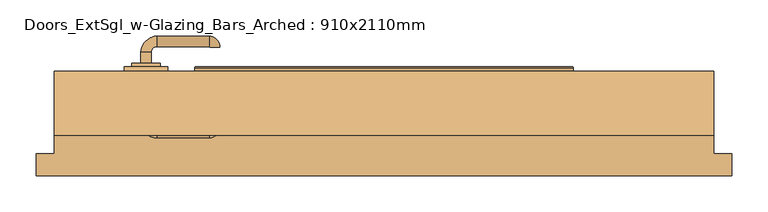
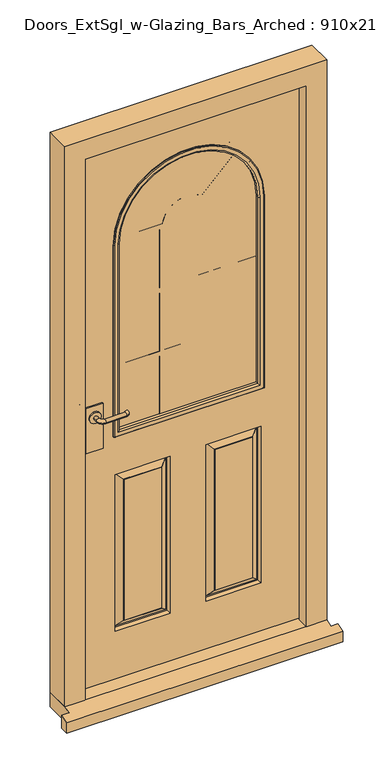
"""IFC4 building model written with IfcOpenShell, lengths in millimetres: door geometry, Doors_ExtSgl_w-Glazing_Bars_Arched : 910x2110mm."""

from ifc_helpers import new_model, si_unit, point, frame, frame_2d, origin, place, context, project, spatial, polyline, circle_curve, ellipse_curve, trimmed, segment, composite_curve, outline, extrude, faceted_brep, source, transform, mapped, element, save
from ifc_brep_helpers import plane_surface, cylinder_surface, revolved_surface, advanced_brep


def doors_extsgl_w_glazing_bars_arched_910x2110mm_97dcda8a(model_context):
    return source(origin(), model_context, "Body", "SolidModel", [
        extrude(outline(composite_curve([segment(trimmed(circle_curve(frame_2d((1050.0, -328.5)), 20.0), [point((1050.0, -348.5))], [point((1050.0, -308.5))], False, "CARTESIAN"), True, "CONTINUOUS"), segment(trimmed(circle_curve(frame_2d((1050.0, -328.5)), 20.0), [point((1050.0, -308.5))], [point((1050.0, -348.5))], False, "CARTESIAN"), True, "CONTINUOUS")], self_intersect=False)), frame((0.0, 18.4, 0.0), z_axis=(0.0, 1.0, 0.0), x_axis=(0.0, 0.0, 1.0)), (0.0, 0.0, 1.0), 4.5929895),
        advanced_brep(
        [(-321.5, 22.9929895, 1050.0), (-335.5, 22.9929895, 1050.0), (-321.5, 38.4, 1050.0), (-335.5, 38.4, 1050.0), (-313.5, 60.4, 1050.0), (-313.5, 46.4, 1050.0), (-241.5, 46.4, 1050.0), (-241.5, 60.4, 1050.0), (-240.5, 45.4, 1050.0), (-226.5, 45.4, 1050.0)],
        [
            (0, 1, circle_curve(frame((-328.5, 22.9929895, 1050.0), z_axis=(0.0, -1.0, 0.0), x_axis=(-1.0, 0.0, 0.0)), 7.0)),
            (1, 0, circle_curve(frame((-328.5, 22.9929895, 1050.0), z_axis=(0.0, -1.0, 0.0), x_axis=(-1.0, 0.0, 0.0)), 7.0)),
            (0, 2),
            (2, 3, circle_curve(frame((-328.5, 38.4, 1050.0), z_axis=(0.0, -1.0, 0.0), x_axis=(-1.0, 0.0, 0.0)), 7.0)),
            (3, 1),
            (3, 2, circle_curve(frame((-328.5, 38.4, 1050.0), z_axis=(0.0, -1.0, 0.0), x_axis=(-1.0, 0.0, 0.0)), 7.0)),
            (4, 3, circle_curve(frame((-313.5, 38.4, 1050.0), z_axis=(0.0, 0.0, 1.0), x_axis=(-1.0, 0.0, 0.0)), 22.0)),
            (2, 5, circle_curve(frame((-313.5, 38.4, 1050.0), z_axis=(0.0, 0.0, -1.0), x_axis=(-1.0, 0.0, 0.0)), 8.0)),
            (5, 4, circle_curve(frame((-313.5, 53.4, 1050.0), z_axis=(-1.0, 0.0, 0.0), x_axis=(0.0, 1.0, 0.0)), 7.0)),
            (4, 5, circle_curve(frame((-313.5, 53.4, 1050.0), z_axis=(-1.0, 0.0, 0.0), x_axis=(0.0, 1.0, 0.0)), 7.0)),
            (5, 6),
            (6, 7, circle_curve(frame((-241.5, 53.4, 1050.0), z_axis=(-1.0, 0.0, 0.0), x_axis=(0.0, 1.0, 0.0)), 7.0)),
            (7, 4),
            (7, 6, circle_curve(frame((-241.5, 53.4, 1050.0), z_axis=(-1.0, 0.0, 0.0), x_axis=(0.0, 1.0, 0.0)), 7.0)),
            (8, 9, circle_curve(frame((-233.5, 45.4, 1050.0), z_axis=(0.0, -1.0, 0.0), x_axis=(1.0, 0.0, 0.0)), 7.0)),
            (9, 8, circle_curve(frame((-233.5, 45.4, 1050.0), z_axis=(0.0, -1.0, 0.0), x_axis=(1.0, 0.0, 0.0)), 7.0)),
            (9, 7, circle_curve(frame((-241.5, 45.4, 1050.0), z_axis=(0.0, 0.0, 1.0), x_axis=(0.0, 1.0, 0.0)), 15.0)),
            (6, 8, circle_curve(frame((-241.5, 45.4, 1050.0), z_axis=(0.0, 0.0, -1.0), x_axis=(0.0, 1.0, 0.0)), 1.0)),
        ],
        [
            plane_surface(frame((-328.5, 22.9929895, 1050.0), z_axis=(0.0, -1.0, 0.0), x_axis=(0.0, 0.0, 1.0))),
            cylinder_surface(frame((-328.5, 22.9929895, 1050.0), z_axis=(0.0, -1.0, 0.0), x_axis=(-1.0, 0.0, 0.0)), 7.0),
            revolved_surface(trimmed(ellipse_curve(frame((-328.5, 38.4, 1050.0), z_axis=(0.0, -1.0, 0.0), x_axis=(-1.0, 0.0, 0.0)), 7.0, 7.0), [point((-321.5, 38.4, 1050.0))], [point((-335.5, 38.4, 1050.0))], True, "CARTESIAN"), (-313.5, 38.4, 1050.0), (0.0, 0.0, -1.0)),
            revolved_surface(trimmed(ellipse_curve(frame((-328.5, 38.4, 1050.0), z_axis=(0.0, -1.0, 0.0), x_axis=(-1.0, 0.0, 0.0)), 7.0, 7.0), [point((-335.5, 38.4, 1050.0))], [point((-321.5, 38.4, 1050.0))], True, "CARTESIAN"), (-313.5, 38.4, 1050.0), (0.0, 0.0, -1.0)),
            cylinder_surface(frame((-313.5, 53.4, 1050.0), z_axis=(-1.0, 0.0, 0.0), x_axis=(0.0, 1.0, 0.0)), 7.0),
            plane_surface(frame((-233.5, 45.4, 1050.0), z_axis=(0.0, -1.0, 0.0), x_axis=(0.0, 0.0, 1.0))),
            revolved_surface(trimmed(ellipse_curve(frame((-241.5, 53.4, 1050.0), z_axis=(-1.0, 0.0, 0.0), x_axis=(0.0, 1.0, 0.0)), 7.0, 7.0), [point((-241.5, 46.4, 1050.0))], [point((-241.5, 60.4, 1050.0))], True, "CARTESIAN"), (-241.5, 45.4, 1050.0), (0.0, 0.0, -1.0)),
            revolved_surface(trimmed(ellipse_curve(frame((-241.5, 53.4, 1050.0), z_axis=(-1.0, 0.0, 0.0), x_axis=(0.0, 1.0, 0.0)), 7.0, 7.0), [point((-241.5, 60.4, 1050.0))], [point((-241.5, 46.4, 1050.0))], True, "CARTESIAN"), (-241.5, 45.4, 1050.0), (0.0, 0.0, -1.0)),
        ],
        [
            (0, [[1, 2]]),
            (1, [[-1, 3, 4, 5]]),
            (1, [[-2, -5, 6, -3]]),
            (2, [[7, -4, 8, 9]]),
            (3, [[-8, -6, -7, 10]]),
            (4, [[-9, 11, 12, 13]]),
            (4, [[-10, -13, 14, -11]]),
            (5, [[15, 16]]),
            (6, [[17, -12, 18, -16]]),
            (7, [[-18, -14, -17, -15]]),
        ],
    ),
        extrude(outline(polyline([(-298.5, 12.4), (-358.5, 12.4), (-358.5, 18.4), (-298.5, 18.4), (-298.5, 12.4)])), frame((0.0, 0.0, 925.0), z_axis=(0.0, 0.0, 1.0), x_axis=(1.0, 0.0, 0.0)), (0.0, 0.0, 1.0), 165.0),
        extrude(outline(composite_curve([segment(trimmed(circle_curve(frame_2d((1050.0, -328.5)), 20.0), [point((1050.0, -348.5))], [point((1050.0, -308.5))], False, "CARTESIAN"), True, "CONTINUOUS"), segment(trimmed(circle_curve(frame_2d((1050.0, -328.5)), 20.0), [point((1050.0, -308.5))], [point((1050.0, -348.5))], False, "CARTESIAN"), True, "CONTINUOUS")], self_intersect=False)), frame((0.0, -42.1929895, 0.0), z_axis=(0.0, 1.0, 0.0), x_axis=(0.0, 0.0, 1.0)), (0.0, 0.0, 1.0), 4.5929895),
        advanced_brep(
        [(-321.5, -42.1929895, 1050.0), (-335.5, -42.1929895, 1050.0), (-335.5, -57.6, 1050.0), (-321.5, -57.6, 1050.0), (-313.5, -79.6, 1050.0), (-313.5, -65.6, 1050.0), (-241.5, -79.6, 1050.0), (-241.5, -65.6, 1050.0), (-240.5, -64.6, 1050.0), (-226.5, -64.6, 1050.0)],
        [
            (0, 1, circle_curve(frame((-328.5, -42.1929895, 1050.0), z_axis=(0.0, 1.0, 0.0), x_axis=(-1.0, 0.0, 0.0)), 7.0)),
            (1, 0, circle_curve(frame((-328.5, -42.1929895, 1050.0), z_axis=(0.0, 1.0, 0.0), x_axis=(-1.0, 0.0, 0.0)), 7.0)),
            (1, 2),
            (2, 3, circle_curve(frame((-328.5, -57.6, 1050.0), z_axis=(0.0, 1.0, 0.0), x_axis=(-1.0, 0.0, 0.0)), 7.0)),
            (3, 0),
            (3, 2, circle_curve(frame((-328.5, -57.6, 1050.0), z_axis=(0.0, 1.0, 0.0), x_axis=(-1.0, 0.0, 0.0)), 7.0)),
            (4, 5, circle_curve(frame((-313.5, -72.6, 1050.0), z_axis=(-1.0, 0.0, 0.0), x_axis=(0.0, -1.0, 0.0)), 7.0)),
            (5, 3, circle_curve(frame((-313.5, -57.6, 1050.0), z_axis=(0.0, 0.0, -1.0), x_axis=(-1.0, 0.0, 0.0)), 8.0)),
            (2, 4, circle_curve(frame((-313.5, -57.6, 1050.0), z_axis=(0.0, 0.0, 1.0), x_axis=(-1.0, 0.0, 0.0)), 22.0)),
            (5, 4, circle_curve(frame((-313.5, -72.6, 1050.0), z_axis=(-1.0, 0.0, 0.0), x_axis=(0.0, -1.0, 0.0)), 7.0)),
            (4, 6),
            (6, 7, circle_curve(frame((-241.5, -72.6, 1050.0), z_axis=(-1.0, 0.0, 0.0), x_axis=(0.0, -1.0, 0.0)), 7.0)),
            (7, 5),
            (7, 6, circle_curve(frame((-241.5, -72.6, 1050.0), z_axis=(-1.0, 0.0, 0.0), x_axis=(0.0, -1.0, 0.0)), 7.0)),
            (8, 9, circle_curve(frame((-233.5, -64.6, 1050.0), z_axis=(0.0, 1.0, 0.0), x_axis=(1.0, 0.0, 0.0)), 7.0)),
            (9, 8, circle_curve(frame((-233.5, -64.6, 1050.0), z_axis=(0.0, 1.0, 0.0), x_axis=(1.0, 0.0, 0.0)), 7.0)),
            (8, 7, circle_curve(frame((-241.5, -64.6, 1050.0), z_axis=(0.0, 0.0, -1.0), x_axis=(0.0, -1.0, 0.0)), 1.0)),
            (6, 9, circle_curve(frame((-241.5, -64.6, 1050.0), z_axis=(0.0, 0.0, 1.0), x_axis=(0.0, -1.0, 0.0)), 15.0)),
        ],
        [
            plane_surface(frame((-328.5, -42.1929895, 1050.0), z_axis=(0.0, 1.0, 0.0), x_axis=(0.0, 0.0, 1.0))),
            cylinder_surface(frame((-328.5, -42.1929895, 1050.0), z_axis=(0.0, 1.0, 0.0), x_axis=(-1.0, 0.0, 0.0)), 7.0),
            revolved_surface(trimmed(ellipse_curve(frame((-328.5, -57.6, 1050.0), z_axis=(0.0, -1.0, 0.0), x_axis=(-1.0, 0.0, 0.0)), 7.0, 7.0), [point((-321.5, -57.6, 1050.0))], [point((-335.5, -57.6, 1050.0))], True, "CARTESIAN"), (-313.5, -57.6, 1050.0), (0.0, 0.0, -1.0)),
            revolved_surface(trimmed(ellipse_curve(frame((-328.5, -57.6, 1050.0), z_axis=(0.0, -1.0, 0.0), x_axis=(-1.0, 0.0, 0.0)), 7.0, 7.0), [point((-335.5, -57.6, 1050.0))], [point((-321.5, -57.6, 1050.0))], True, "CARTESIAN"), (-313.5, -57.6, 1050.0), (0.0, 0.0, -1.0)),
            cylinder_surface(frame((-313.5, -72.6, 1050.0), z_axis=(-1.0, 0.0, 0.0), x_axis=(0.0, -1.0, 0.0)), 7.0),
            plane_surface(frame((-233.5, -64.6, 1050.0), z_axis=(0.0, 1.0, 0.0), x_axis=(0.0, 0.0, 1.0))),
            revolved_surface(trimmed(ellipse_curve(frame((-241.5, -72.6, 1050.0), z_axis=(1.0, 0.0, 0.0), x_axis=(0.0, -1.0, 0.0)), 7.0, 7.0), [point((-241.5, -65.6, 1050.0))], [point((-241.5, -79.6, 1050.0))], True, "CARTESIAN"), (-241.5, -64.6, 1050.0), (0.0, 0.0, -1.0)),
            revolved_surface(trimmed(ellipse_curve(frame((-241.5, -72.6, 1050.0), z_axis=(1.0, 0.0, 0.0), x_axis=(0.0, -1.0, 0.0)), 7.0, 7.0), [point((-241.5, -79.6, 1050.0))], [point((-241.5, -65.6, 1050.0))], True, "CARTESIAN"), (-241.5, -64.6, 1050.0), (0.0, 0.0, -1.0)),
        ],
        [
            (0, [[1, 2]]),
            (1, [[3, 4, 5, -2]]),
            (1, [[-5, 6, -3, -1]]),
            (2, [[7, 8, -4, 9]]),
            (3, [[10, -9, -6, -8]]),
            (4, [[11, 12, 13, -7]]),
            (4, [[-13, 14, -11, -10]]),
            (5, [[15, 16]]),
            (6, [[-15, 17, -12, 18]]),
            (7, [[-16, -18, -14, -17]]),
        ],
    ),
        extrude(outline(polyline([(-298.5, -31.6), (-298.5, -37.6), (-358.5, -37.6), (-358.5, -31.6), (-298.5, -31.6)])), frame((0.0, 0.0, 925.0), z_axis=(0.0, 0.0, 1.0), x_axis=(1.0, 0.0, 0.0)), (0.0, 0.0, 1.0), 165.0),
        faceted_brep([(384.5, -76.6, 54.5), (384.5, -34.6, 54.5), (406.5, -34.6, 54.5), (406.5, 12.4, 54.5), (455.0, 12.4, 54.5), (455.0, -76.6, 54.5), (455.0, -76.6, 2110.0), (-455.0, -76.6, 2110.0), (-455.0, -76.6, 54.5), (-384.5, -76.6, 54.5), (-384.5, -76.6, 2039.5), (384.5, -76.6, 2039.5), (455.0, 12.4, 2110.0), (406.5, 12.4, 2061.5), (-406.5, 12.4, 2061.5), (-406.5, 12.4, 54.5), (-455.0, 12.4, 54.5), (-455.0, 12.4, 2110.0), (406.5, -34.6, 2061.5), (384.5, -34.6, 2039.5), (-384.5, -34.6, 2039.5), (-384.5, -34.6, 54.5), (-406.5, -34.6, 54.5), (-406.5, -34.6, 2061.5)], [[[0, 1, 2, 3, 4, 5]], [[5, 6, 7, 8, 9, 10, 11, 0]], [[4, 12, 6, 5]], [[3, 13, 14, 15, 16, 17, 12, 4]], [[2, 18, 13, 3]], [[1, 19, 20, 21, 22, 23, 18, 2]], [[0, 11, 19, 1]], [[9, 21, 20, 10]], [[8, 16, 15, 22, 21, 9]], [[7, 17, 16, 8]], [[14, 23, 22, 15]], [[6, 12, 17, 7]], [[13, 18, 23, 14]], [[10, 20, 19, 11]]]),
        advanced_brep(
        [(403.5, 12.4, 58.5), (-404.4250294, 12.4, 58.5), (-404.4250294, 12.4, 2058.5), (403.5, 12.4, 2058.5), (-253.5, 12.4, 958.5), (253.5, 12.4, 958.5), (253.5, 12.4, 1655.0), (-253.5, 12.4, 1655.0), (-62.5, 12.4, 808.5), (-253.5, 12.4, 808.5), (-253.5, 12.4, 233.5), (-62.5, 12.4, 233.5), (253.5, 12.4, 808.5), (62.5, 12.4, 808.5), (62.5, 12.4, 233.5), (253.5, 12.4, 233.5), (-92.5, 12.4, 263.5), (-223.5, 12.4, 263.5), (-223.5, 12.4, 778.5), (-92.5, 12.4, 778.5), (223.5, 12.4, 263.5), (92.5, 12.4, 263.5), (92.5, 12.4, 778.5), (223.5, 12.4, 778.5), (403.5, -31.6, 58.5), (403.5, -31.6, 2058.5), (-404.4250294, -31.6, 2058.5), (-404.4250294, -31.6, 58.5), (-253.5, -31.6, 958.5), (-253.5, -31.6, 1655.0), (253.5, -31.6, 1655.0), (253.5, -31.6, 958.5), (62.5, -31.6, 808.5), (253.5, -31.6, 808.5), (253.5, -31.6, 233.5), (62.5, -31.6, 233.5), (-253.5, -31.6, 808.5), (-62.5, -31.6, 808.5), (-62.5, -31.6, 233.5), (-253.5, -31.6, 233.5), (92.5, -31.6, 263.5), (223.5, -31.6, 263.5), (223.5, -31.6, 778.5), (92.5, -31.6, 778.5), (-223.5, -31.6, 263.5), (-92.5, -31.6, 263.5), (-92.5, -31.6, 778.5), (-223.5, -31.6, 778.5), (65.5, -16.6, 805.5), (65.5, -16.6, 236.5), (90.5, -30.6, 780.5), (70.5, -16.6, 800.5), (70.5, -16.6, 241.5), (90.5, -30.6, 261.5), (92.5, -30.6, 778.5), (92.5, -30.6, 263.5), (250.5, -16.6, 236.5), (245.5, -16.6, 241.5), (225.5, -30.6, 261.5), (223.5, -30.6, 263.5), (250.5, -16.6, 805.5), (245.5, -16.6, 800.5), (225.5, -30.6, 780.5), (223.5, -30.6, 778.5), (-250.5, -16.6, 805.5), (-250.5, -16.6, 236.5), (-225.5, -30.6, 780.5), (-245.5, -16.6, 800.5), (-245.5, -16.6, 241.5), (-225.5, -30.6, 261.5), (-223.5, -30.6, 778.5), (-223.5, -30.6, 263.5), (-65.5, -16.6, 236.5), (-70.5, -16.6, 241.5), (-90.5, -30.6, 261.5), (-92.5, -30.6, 263.5), (-65.5, -16.6, 805.5), (-70.5, -16.6, 800.5), (-90.5, -30.6, 780.5), (-92.5, -30.6, 778.5), (-92.5, 11.4, 263.5), (-92.5, 11.4, 778.5), (-70.5, -2.6, 241.5), (-90.5, 11.4, 261.5), (-90.5, 11.4, 780.5), (-70.5, -2.6, 800.5), (-65.5, -2.6, 236.5), (-65.5, -2.6, 805.5), (-223.5, 11.4, 778.5), (-225.5, 11.4, 780.5), (-245.5, -2.6, 800.5), (-250.5, -2.6, 805.5), (-223.5, 11.4, 263.5), (-225.5, 11.4, 261.5), (-245.5, -2.6, 241.5), (-250.5, -2.6, 236.5), (250.5, -2.6, 805.5), (250.5, -2.6, 236.5), (225.5, 11.4, 780.5), (245.5, -2.6, 800.5), (245.5, -2.6, 241.5), (225.5, 11.4, 261.5), (223.5, 11.4, 778.5), (223.5, 11.4, 263.5), (65.5, -2.6, 236.5), (70.5, -2.6, 241.5), (90.5, 11.4, 261.5), (92.5, 11.4, 263.5), (65.5, -2.6, 805.5), (70.5, -2.6, 800.5), (90.5, 11.4, 780.5), (92.5, 11.4, 778.5)],
        [
            (0, 1),
            (1, 2),
            (2, 3),
            (3, 0),
            (4, 5),
            (5, 6),
            (6, 7, circle_curve(frame((0.0, 12.4, 1655.0), z_axis=(0.0, -1.0, 0.0), x_axis=(1.0, 0.0, 0.0)), 253.5)),
            (7, 4),
            (8, 9),
            (9, 10),
            (10, 11),
            (11, 8),
            (12, 13),
            (13, 14),
            (14, 15),
            (15, 12),
            (16, 17),
            (17, 18),
            (18, 19),
            (19, 16),
            (20, 21),
            (21, 22),
            (22, 23),
            (23, 20),
            (24, 25),
            (25, 26),
            (26, 27),
            (27, 24),
            (28, 29),
            (29, 30, circle_curve(frame((0.0, -31.6, 1655.0), z_axis=(0.0, 1.0, 0.0), x_axis=(1.0, 0.0, 0.0)), 253.5)),
            (30, 31),
            (31, 28),
            (32, 33),
            (33, 34),
            (34, 35),
            (35, 32),
            (36, 37),
            (37, 38),
            (38, 39),
            (39, 36),
            (40, 41),
            (41, 42),
            (42, 43),
            (43, 40),
            (44, 45),
            (45, 46),
            (46, 47),
            (47, 44),
            (3, 25),
            (24, 0),
            (2, 26),
            (1, 27),
            (7, 29),
            (28, 4),
            (6, 30),
            (5, 31),
            (48, 32),
            (35, 49),
            (49, 48),
            (50, 51),
            (51, 52),
            (52, 53),
            (53, 50),
            (43, 54),
            (54, 55),
            (55, 40),
            (34, 56),
            (56, 49),
            (52, 57),
            (57, 58),
            (58, 53),
            (55, 59),
            (59, 41),
            (33, 60),
            (60, 56),
            (57, 61),
            (61, 62),
            (62, 58),
            (59, 63),
            (63, 42),
            (48, 60),
            (51, 61),
            (50, 62),
            (54, 63),
            (64, 36),
            (39, 65),
            (65, 64),
            (66, 67),
            (67, 68),
            (68, 69),
            (69, 66),
            (47, 70),
            (70, 71),
            (71, 44),
            (38, 72),
            (72, 65),
            (68, 73),
            (73, 74),
            (74, 69),
            (71, 75),
            (75, 45),
            (37, 76),
            (76, 72),
            (73, 77),
            (77, 78),
            (78, 74),
            (75, 79),
            (79, 46),
            (64, 76),
            (67, 77),
            (66, 78),
            (70, 79),
            (80, 16),
            (19, 81),
            (81, 80),
            (82, 83),
            (83, 84),
            (84, 85),
            (85, 82),
            (11, 86),
            (86, 87),
            (87, 8),
            (18, 88),
            (88, 81),
            (84, 89),
            (89, 90),
            (90, 85),
            (87, 91),
            (91, 9),
            (17, 92),
            (92, 88),
            (89, 93),
            (93, 94),
            (94, 90),
            (91, 95),
            (95, 10),
            (80, 92),
            (83, 93),
            (82, 94),
            (86, 95),
            (96, 12),
            (15, 97),
            (97, 96),
            (98, 99),
            (99, 100),
            (100, 101),
            (101, 98),
            (23, 102),
            (102, 103),
            (103, 20),
            (14, 104),
            (104, 97),
            (100, 105),
            (105, 106),
            (106, 101),
            (103, 107),
            (107, 21),
            (13, 108),
            (108, 104),
            (105, 109),
            (109, 110),
            (110, 106),
            (107, 111),
            (111, 22),
            (96, 108),
            (99, 109),
            (98, 110),
            (102, 111),
        ],
        [
            plane_surface(frame((403.5, 12.4, 58.5), z_axis=(0.0, 1.0, 0.0), x_axis=(0.0, 0.0, 1.0))),
            plane_surface(frame((403.5, -31.6, 58.5), z_axis=(0.0, -1.0, 0.0), x_axis=(0.0, 0.0, -1.0))),
            plane_surface(frame((403.5, 12.4, 58.5), z_axis=(1.0, 0.0, 0.0), x_axis=(0.0, -1.0, 0.0))),
            plane_surface(frame((403.5, 12.4, 2058.5), z_axis=(0.0, 0.0, 1.0), x_axis=(0.0, -1.0, 0.0))),
            plane_surface(frame((-404.4250294, 12.4, 2058.5), z_axis=(-1.0, 0.0, 0.0), x_axis=(0.0, -1.0, 0.0))),
            plane_surface(frame((-404.4250294, 12.4, 58.5), z_axis=(0.0, 0.0, -1.0), x_axis=(0.0, -1.0, 0.0))),
            plane_surface(frame((-253.5, 12.4, 958.5), z_axis=(1.0, 0.0, 0.0), x_axis=(0.0, -1.0, 0.0))),
            revolved_surface(polyline([(253.5, -31.6, 1655.0), (253.5, 12.4, 1655.0)]), (0.0, 12.4, 1655.0), (0.0, -1.0, 0.0)),
            plane_surface(frame((253.5, 12.4, 1655.0), z_axis=(-1.0, 0.0, 0.0), x_axis=(0.0, -1.0, 0.0))),
            plane_surface(frame((253.5, 12.4, 958.5), z_axis=(0.0, 0.0, 1.0), x_axis=(0.0, -1.0, 0.0))),
            plane_surface(frame((62.5, -31.6, 808.5), z_axis=(0.9805806756909202, -0.19611613513818407, 0.0), x_axis=(0.0, 0.0, -1.0))),
            plane_surface(frame((70.5, -16.6, 800.5), z_axis=(-0.5734623443633278, -0.8192319205190408, 0.0), x_axis=(0.0, 0.0, -1.0))),
            plane_surface(frame((92.5, -30.6, 778.5), z_axis=(-1.0, 0.0, 0.0), x_axis=(0.0, 0.0, -1.0))),
            plane_surface(frame((62.5, -31.6, 233.5), z_axis=(0.0, -0.19611613513818724, 0.9805806756909196), x_axis=(1.0, 0.0, 0.0))),
            plane_surface(frame((70.5, -16.6, 241.5), z_axis=(0.0, -0.819231920519039, -0.5734623443633305), x_axis=(1.0, 0.0, 0.0))),
            plane_surface(frame((92.5, -30.6, 263.5), z_axis=(0.0, 0.0, -1.0), x_axis=(1.0, 0.0, 0.0))),
            plane_surface(frame((253.5, -31.6, 233.5), z_axis=(-0.9805806756909189, -0.19611613513819037, 0.0), x_axis=(0.0, 0.0, 1.0))),
            plane_surface(frame((245.5, -16.6, 241.5), z_axis=(0.5734623443633332, -0.819231920519037, 0.0), x_axis=(0.0, 0.0, 1.0))),
            plane_surface(frame((223.5, -30.6, 263.5), z_axis=(1.0, 0.0, 0.0), x_axis=(0.0, 0.0, 1.0))),
            plane_surface(frame((253.5, -31.6, 808.5), z_axis=(0.0, -0.1961161351381872, -0.9805806756909196), x_axis=(-1.0, 0.0, 0.0))),
            plane_surface(frame((250.5, -16.6, 805.5), z_axis=(0.0, -1.0, 0.0), x_axis=(-1.0, 0.0, 0.0))),
            plane_surface(frame((245.5, -16.6, 800.5), z_axis=(0.0, -0.8192319205190389, 0.5734623443633305), x_axis=(-1.0, 0.0, 0.0))),
            plane_surface(frame((225.5, -30.6, 780.5), z_axis=(0.0, -1.0, 0.0), x_axis=(-1.0, 0.0, 0.0))),
            plane_surface(frame((223.5, -30.6, 778.5), z_axis=(0.0, 0.0, 1.0), x_axis=(-1.0, 0.0, 0.0))),
            plane_surface(frame((-253.5, -31.6, 808.5), z_axis=(0.9805806756909202, -0.19611613513818407, 0.0), x_axis=(0.0, 0.0, -1.0))),
            plane_surface(frame((-245.5, -16.6, 800.5), z_axis=(-0.5734623443633278, -0.8192319205190408, 0.0), x_axis=(0.0, 0.0, -1.0))),
            plane_surface(frame((-223.5, -30.6, 778.5), z_axis=(-1.0, 0.0, 0.0), x_axis=(0.0, 0.0, -1.0))),
            plane_surface(frame((-253.5, -31.6, 233.5), z_axis=(0.0, -0.19611613513818724, 0.9805806756909196), x_axis=(1.0, 0.0, 0.0))),
            plane_surface(frame((-245.5, -16.6, 241.5), z_axis=(0.0, -0.819231920519039, -0.5734623443633305), x_axis=(1.0, 0.0, 0.0))),
            plane_surface(frame((-223.5, -30.6, 263.5), z_axis=(0.0, 0.0, -1.0), x_axis=(1.0, 0.0, 0.0))),
            plane_surface(frame((-62.5, -31.6, 233.5), z_axis=(-0.9805806756909189, -0.1961161351381904, 0.0), x_axis=(0.0, 0.0, 1.0))),
            plane_surface(frame((-70.5, -16.6, 241.5), z_axis=(0.5734623443633332, -0.8192319205190371, 0.0), x_axis=(0.0, 0.0, 1.0))),
            plane_surface(frame((-92.5, -30.6, 263.5), z_axis=(1.0, 0.0, 0.0), x_axis=(0.0, 0.0, 1.0))),
            plane_surface(frame((-62.5, -31.6, 808.5), z_axis=(0.0, -0.19611613513818724, -0.9805806756909196), x_axis=(-1.0, 0.0, 0.0))),
            plane_surface(frame((-65.5, -16.6, 805.5), z_axis=(0.0, -1.0, 0.0), x_axis=(-1.0, 0.0, 0.0))),
            plane_surface(frame((-70.5, -16.6, 800.5), z_axis=(0.0, -0.819231920519039, 0.5734623443633305), x_axis=(-1.0, 0.0, 0.0))),
            plane_surface(frame((-90.5, -30.6, 780.5), z_axis=(0.0, -1.0, 0.0), x_axis=(-1.0, 0.0, 0.0))),
            plane_surface(frame((-92.5, -30.6, 778.5), z_axis=(0.0, 0.0, 1.0), x_axis=(-1.0, 0.0, 0.0))),
            plane_surface(frame((-92.5, 12.4, 263.5), z_axis=(1.0, 0.0, 0.0), x_axis=(0.0, 0.0, 1.0))),
            plane_surface(frame((-90.5, 11.4, 261.5), z_axis=(0.5734623443633226, 0.8192319205190446, 0.0), x_axis=(0.0, 0.0, 1.0))),
            plane_surface(frame((-65.5, -2.6, 236.5), z_axis=(-0.9805806756909214, 0.19611613513817774, 0.0), x_axis=(0.0, 0.0, 1.0))),
            plane_surface(frame((-92.5, 12.4, 778.5), z_axis=(0.0, 0.0, 1.0), x_axis=(-1.0, 0.0, 0.0))),
            plane_surface(frame((-90.5, 11.4, 780.5), z_axis=(0.0, 0.8192319205190427, 0.5734623443633252), x_axis=(-1.0, 0.0, 0.0))),
            plane_surface(frame((-65.5, -2.6, 805.5), z_axis=(0.0, 0.1961161351381809, -0.9805806756909208), x_axis=(-1.0, 0.0, 0.0))),
            plane_surface(frame((-223.5, 12.4, 778.5), z_axis=(-1.0, 0.0, 0.0), x_axis=(0.0, 0.0, -1.0))),
            plane_surface(frame((-225.5, 11.4, 780.5), z_axis=(-0.5734623443633279, 0.8192319205190408, 0.0), x_axis=(0.0, 0.0, -1.0))),
            plane_surface(frame((-250.5, -2.6, 805.5), z_axis=(0.9805806756909202, 0.1961161351381841, 0.0), x_axis=(0.0, 0.0, -1.0))),
            plane_surface(frame((-223.5, 12.4, 263.5), z_axis=(0.0, 0.0, -1.0), x_axis=(1.0, 0.0, 0.0))),
            plane_surface(frame((-223.5, 11.4, 263.5), z_axis=(0.0, 1.0, 0.0), x_axis=(1.0, 0.0, 0.0))),
            plane_surface(frame((-225.5, 11.4, 261.5), z_axis=(0.0, 0.8192319205190427, -0.5734623443633252), x_axis=(1.0, 0.0, 0.0))),
            plane_surface(frame((-245.5, -2.6, 241.5), z_axis=(0.0, 1.0, 0.0), x_axis=(1.0, 0.0, 0.0))),
            plane_surface(frame((-250.5, -2.6, 236.5), z_axis=(0.0, 0.19611613513818094, 0.9805806756909209), x_axis=(1.0, 0.0, 0.0))),
            plane_surface(frame((253.5, 12.4, 808.5), z_axis=(-0.9805806756909202, 0.19611613513818407, 0.0), x_axis=(0.0, 0.0, -1.0))),
            plane_surface(frame((245.5, -2.6, 800.5), z_axis=(0.5734623443633278, 0.8192319205190408, 0.0), x_axis=(0.0, 0.0, -1.0))),
            plane_surface(frame((223.5, 11.4, 778.5), z_axis=(1.0, 0.0, 0.0), x_axis=(0.0, 0.0, -1.0))),
            plane_surface(frame((253.5, 12.4, 233.5), z_axis=(0.0, 0.19611613513818724, 0.9805806756909196), x_axis=(-1.0, 0.0, 0.0))),
            plane_surface(frame((245.5, -2.6, 241.5), z_axis=(0.0, 0.819231920519039, -0.5734623443633305), x_axis=(-1.0, 0.0, 0.0))),
            plane_surface(frame((223.5, 11.4, 263.5), z_axis=(0.0, 0.0, -1.0), x_axis=(-1.0, 0.0, 0.0))),
            plane_surface(frame((62.5, 12.4, 233.5), z_axis=(0.9805806756909189, 0.19611613513819046, 0.0), x_axis=(0.0, 0.0, 1.0))),
            plane_surface(frame((70.5, -2.6, 241.5), z_axis=(-0.5734623443633331, 0.8192319205190371, 0.0), x_axis=(0.0, 0.0, 1.0))),
            plane_surface(frame((92.5, 11.4, 263.5), z_axis=(-1.0, 0.0, 0.0), x_axis=(0.0, 0.0, 1.0))),
            plane_surface(frame((62.5, 12.4, 808.5), z_axis=(0.0, 0.1961161351381873, -0.9805806756909196), x_axis=(1.0, 0.0, 0.0))),
            plane_surface(frame((65.5, -2.6, 805.5), z_axis=(0.0, 1.0, 0.0), x_axis=(1.0, 0.0, 0.0))),
            plane_surface(frame((70.5, -2.6, 800.5), z_axis=(0.0, 0.819231920519039, 0.5734623443633304), x_axis=(1.0, 0.0, 0.0))),
            plane_surface(frame((90.5, 11.4, 780.5), z_axis=(0.0, 1.0, 0.0), x_axis=(1.0, 0.0, 0.0))),
            plane_surface(frame((92.5, 11.4, 778.5), z_axis=(0.0, 0.0, 1.0), x_axis=(1.0, 0.0, 0.0))),
        ],
        [
            (0, [[1, 2, 3, 4], [5, 6, 7, 8], [9, 10, 11, 12], [13, 14, 15, 16]]),
            (0, [[17, 18, 19, 20]]),
            (0, [[21, 22, 23, 24]]),
            (1, [[25, 26, 27, 28], [29, 30, 31, 32], [33, 34, 35, 36], [37, 38, 39, 40]]),
            (1, [[41, 42, 43, 44]]),
            (1, [[45, 46, 47, 48]]),
            (2, [[49, -25, 50, -4]]),
            (3, [[51, -26, -49, -3]]),
            (4, [[52, -27, -51, -2]]),
            (5, [[-50, -28, -52, -1]]),
            (6, [[53, -29, 54, -8]]),
            (7, [[55, -30, -53, -7]]),
            (8, [[56, -31, -55, -6]]),
            (9, [[-54, -32, -56, -5]]),
            (10, [[57, -36, 58, 59]]),
            (11, [[60, 61, 62, 63]]),
            (12, [[-44, 64, 65, 66]]),
            (13, [[-35, 67, 68, -58]]),
            (14, [[69, 70, 71, -62]]),
            (15, [[72, 73, -41, -66]]),
            (16, [[-34, 74, 75, -67]]),
            (17, [[76, 77, 78, -70]]),
            (18, [[79, 80, -42, -73]]),
            (19, [[81, -74, -33, -57]]),
            (20, [[-68, -75, -81, -59], [82, -76, -69, -61]]),
            (21, [[83, -77, -82, -60]]),
            (22, [[-71, -78, -83, -63], [84, -79, -72, -65]]),
            (23, [[-43, -80, -84, -64]]),
            (24, [[85, -40, 86, 87]]),
            (25, [[88, 89, 90, 91]]),
            (26, [[-48, 92, 93, 94]]),
            (27, [[-39, 95, 96, -86]]),
            (28, [[97, 98, 99, -90]]),
            (29, [[100, 101, -45, -94]]),
            (30, [[-38, 102, 103, -95]]),
            (31, [[104, 105, 106, -98]]),
            (32, [[107, 108, -46, -101]]),
            (33, [[109, -102, -37, -85]]),
            (34, [[-96, -103, -109, -87], [110, -104, -97, -89]]),
            (35, [[111, -105, -110, -88]]),
            (36, [[-99, -106, -111, -91], [112, -107, -100, -93]]),
            (37, [[-47, -108, -112, -92]]),
            (38, [[113, -20, 114, 115]]),
            (39, [[116, 117, 118, 119]]),
            (40, [[-12, 120, 121, 122]]),
            (41, [[-19, 123, 124, -114]]),
            (42, [[125, 126, 127, -118]]),
            (43, [[128, 129, -9, -122]]),
            (44, [[-18, 130, 131, -123]]),
            (45, [[132, 133, 134, -126]]),
            (46, [[135, 136, -10, -129]]),
            (47, [[137, -130, -17, -113]]),
            (48, [[138, -132, -125, -117], [-124, -131, -137, -115]]),
            (49, [[139, -133, -138, -116]]),
            (50, [[140, -135, -128, -121], [-127, -134, -139, -119]]),
            (51, [[-11, -136, -140, -120]]),
            (52, [[141, -16, 142, 143]]),
            (53, [[144, 145, 146, 147]]),
            (54, [[-24, 148, 149, 150]]),
            (55, [[-15, 151, 152, -142]]),
            (56, [[153, 154, 155, -146]]),
            (57, [[156, 157, -21, -150]]),
            (58, [[-14, 158, 159, -151]]),
            (59, [[160, 161, 162, -154]]),
            (60, [[163, 164, -22, -157]]),
            (61, [[165, -158, -13, -141]]),
            (62, [[-152, -159, -165, -143], [166, -160, -153, -145]]),
            (63, [[167, -161, -166, -144]]),
            (64, [[-155, -162, -167, -147], [168, -163, -156, -149]]),
            (65, [[-23, -164, -168, -148]]),
        ],
    ),
        faceted_brep([(480.0, -131.6, 0.0), (480.0, -101.6, 0.0), (480.0, -101.6, 47.2703282), (480.0, -131.6, 38.5947221), (-480.0, -131.6, 38.5947221), (-480.0, -101.6, 47.2703282), (-480.0, -101.6, 0.0), (-480.0, -131.6, 0.0), (-455.0, -101.6, 0.0), (-455.0, 12.4, 0.0), (455.0, 12.4, 0.0), (455.0, -101.6, 0.0), (455.0, -101.6, 47.2703282), (455.0, -76.6, 54.5), (-455.0, -76.6, 54.5), (-455.0, -101.6, 47.2703282), (455.0, 12.4, 54.5), (-455.0, 12.4, 54.5)], [[[0, 1, 2, 3]], [[4, 5, 6, 7]], [[7, 6, 8, 9, 10, 11, 1, 0]], [[3, 4, 7, 0]], [[3, 2, 12, 13, 14, 15, 5, 4]], [[14, 13, 16, 17]], [[17, 16, 10, 9]], [[15, 14, 17, 9, 8]], [[8, 6, 5, 15]], [[11, 10, 16, 13, 12]], [[12, 2, 1, 11]]]),
        extrude(outline(composite_curve([segment(polyline([(958.5, -253.5), (958.5, 253.5), (1655.0, 253.5)]), True, "CONTINUOUS"), segment(trimmed(circle_curve(frame_2d((1655.0, 0.0)), 253.5), [point((1655.0, 253.5))], [point((1655.0, -253.5))], False, "CARTESIAN"), True, "CONTINUOUS"), segment(polyline([(1655.0, -253.5), (958.5, -253.5)]), True, "CONTINUOUS")], self_intersect=False)), frame((0.0, -21.6, 0.0), z_axis=(0.0, 1.0, 0.0), x_axis=(0.0, 0.0, 1.0)), (0.0, 0.0, 1.0), 24.0),
        advanced_brep(
        [(-261.5, -35.6, 950.5), (-261.5, -35.6, 1655.0), (-261.5, -31.6, 1655.0), (-261.5, -31.6, 950.5), (-259.5, -37.6, 952.5), (-259.5, -37.6, 1655.0), (-241.5, -32.6, 970.5), (-241.5, -32.6, 1655.0), (-246.5, -37.6, 1655.0), (-246.5, -37.6, 965.5), (-241.5, -21.6, 970.5), (-241.5, -21.6, 1655.0), (-253.5, -31.6, 958.5), (-253.5, -31.6, 1655.0), (-253.5, -21.6, 1655.0), (-253.5, -21.6, 958.5), (261.5, -35.6, 1655.0), (261.5, -31.6, 1655.0), (259.5, -37.6, 1655.0), (259.5, -37.6, 952.5), (246.5, -37.6, 1655.0), (246.5, -37.6, 965.5), (241.5, -32.6, 1655.0), (241.5, -21.6, 1655.0), (253.5, -21.6, 1655.0), (253.5, -21.6, 958.5), (241.5, -21.6, 970.5), (253.5, -31.6, 1655.0), (261.5, -31.6, 950.5), (253.5, -31.6, 958.5), (261.5, -35.6, 950.5), (241.5, -32.6, 970.5)],
        [
            (0, 1),
            (1, 2),
            (2, 3),
            (3, 0),
            (4, 5),
            (5, 1, circle_curve(frame((-259.5, -35.6, 1655.0), z_axis=(0.0, 0.0, -1.0), x_axis=(-1.0, 0.0, 0.0)), 2.0)),
            (0, 4, ellipse_curve(frame((-259.5, -35.6, 952.5), z_axis=(-0.7071067811865475, 0.0, 0.7071067811865475), x_axis=(-0.7071067811865472, 0.0, -0.7071067811865477)), 2.8284271, 2.0)),
            (6, 7),
            (7, 8, circle_curve(frame((-246.5, -32.6, 1655.0), z_axis=(0.0, 0.0, -1.0), x_axis=(-1.0, 0.0, 0.0)), 5.0)),
            (8, 9),
            (9, 6, ellipse_curve(frame((-246.5, -32.6, 965.5), z_axis=(-0.7071067811865475, 0.0, 0.7071067811865475), x_axis=(-0.7071067811865472, 0.0, -0.7071067811865477)), 7.0710678, 5.0)),
            (10, 11),
            (11, 7),
            (6, 10),
            (12, 13),
            (13, 14),
            (14, 15),
            (15, 12),
            (16, 17),
            (17, 2, circle_curve(frame((0.0, -31.6, 1655.0), z_axis=(0.0, -1.0, 0.0), x_axis=(-1.0, 0.0, 0.0)), 261.5)),
            (1, 16, circle_curve(frame((0.0, -35.6, 1655.0), z_axis=(0.0, 1.0, 0.0), x_axis=(-1.0, 0.0, 0.0)), 261.5)),
            (18, 16, circle_curve(frame((259.5, -35.6, 1655.0), z_axis=(0.0, 0.0, 1.0), x_axis=(1.0, 0.0, 0.0)), 2.0)),
            (5, 18, circle_curve(frame((0.0, -37.6, 1655.0), z_axis=(0.0, 1.0, 0.0), x_axis=(-1.0, 0.0, 0.0)), 259.5)),
            (4, 19),
            (19, 18),
            (20, 21),
            (21, 9),
            (8, 20, circle_curve(frame((0.0, -37.6, 1655.0), z_axis=(0.0, 1.0, 0.0), x_axis=(-1.0, 0.0, 0.0)), 246.5)),
            (22, 20, circle_curve(frame((246.5, -32.6, 1655.0), z_axis=(0.0, 0.0, 1.0), x_axis=(1.0, 0.0, 0.0)), 5.0)),
            (7, 22, circle_curve(frame((0.0, -32.6, 1655.0), z_axis=(0.0, 1.0, 0.0), x_axis=(-1.0, 0.0, 0.0)), 241.5)),
            (23, 22),
            (11, 23, circle_curve(frame((0.0, -21.6, 1655.0), z_axis=(0.0, 1.0, 0.0), x_axis=(-1.0, 0.0, 0.0)), 241.5)),
            (24, 25),
            (25, 15),
            (14, 24, circle_curve(frame((0.0, -21.6, 1655.0), z_axis=(0.0, 1.0, 0.0), x_axis=(-1.0, 0.0, 0.0)), 253.5)),
            (10, 26),
            (26, 23),
            (27, 24),
            (13, 27, circle_curve(frame((0.0, -31.6, 1655.0), z_axis=(0.0, 1.0, 0.0), x_axis=(-1.0, 0.0, 0.0)), 253.5)),
            (17, 28),
            (28, 3),
            (12, 29),
            (29, 27),
            (16, 30),
            (30, 28),
            (19, 30, ellipse_curve(frame((259.5, -35.6, 952.5), z_axis=(0.7071067811865475, 0.0, 0.7071067811865475), x_axis=(-0.7071067811865475, 0.0, 0.7071067811865476)), 2.8284271, 2.0)),
            (22, 31),
            (31, 21, ellipse_curve(frame((246.5, -32.6, 965.5), z_axis=(0.7071067811865475, 0.0, 0.7071067811865475), x_axis=(-0.7071067811865475, 0.0, 0.7071067811865476)), 7.0710678, 5.0)),
            (26, 31),
            (29, 25),
            (30, 0),
            (31, 6),
        ],
        [
            plane_surface(frame((-261.5, -31.6, 950.5), z_axis=(-1.0, 0.0, 0.0), x_axis=(0.0, 0.0, 1.0))),
            cylinder_surface(frame((-259.5, -35.6, 958.5), z_axis=(0.0, 0.0, -1.0), x_axis=(-1.0, 0.0, 0.0)), 2.0),
            cylinder_surface(frame((-246.5, -32.6, 958.5), z_axis=(0.0, 0.0, -1.0), x_axis=(-1.0, 0.0, 0.0)), 5.0),
            plane_surface(frame((-241.5, -32.6, 970.5), z_axis=(1.0, 0.0, 0.0), x_axis=(0.0, 0.0, 1.0))),
            plane_surface(frame((-253.5, -21.6, 958.5), z_axis=(-1.0, 0.0, 0.0), x_axis=(0.0, 0.0, 1.0))),
            cylinder_surface(frame((0.0, -31.6, 1655.0), z_axis=(0.0, -1.0, 0.0), x_axis=(-1.0, 0.0, 0.0)), 261.5),
            revolved_surface(trimmed(ellipse_curve(frame((-259.5, -35.6, 1655.0), z_axis=(0.0, 0.0, 1.0), x_axis=(-1.0, 0.0, 0.0)), 2.0, 2.0), [point((-261.5, -35.6, 1655.0))], [point((-259.5, -37.6, 1655.0))], True, "CARTESIAN"), (0.0, -31.6, 1655.0), (0.0, -1.0, 0.0)),
            plane_surface(frame((0.0, -37.6, 1655.0), z_axis=(0.0, -1.0, 0.0), x_axis=(-1.0, 0.0, 0.0))),
            revolved_surface(trimmed(ellipse_curve(frame((-246.5, -32.6, 1655.0), z_axis=(0.0, 0.0, 1.0), x_axis=(-1.0, 0.0, 0.0)), 5.0, 5.0), [point((-246.5, -37.6, 1655.0))], [point((-241.5, -32.6, 1655.0))], True, "CARTESIAN"), (0.0, -31.6, 1655.0), (0.0, -1.0, 0.0)),
            revolved_surface(polyline([(-241.5, -32.6, 1655.0), (-241.5, -21.6, 1655.0)]), (0.0, -31.6, 1655.0), (0.0, -1.0, 0.0)),
            plane_surface(frame((0.0, -21.6, 1655.0), z_axis=(0.0, 1.0, 0.0), x_axis=(-1.0, 0.0, 0.0))),
            cylinder_surface(frame((0.0, -31.6, 1655.0), z_axis=(0.0, -1.0, 0.0), x_axis=(-1.0, 0.0, 0.0)), 253.5),
            plane_surface(frame((0.0, -31.6, 1655.0), z_axis=(0.0, 1.0, 0.0), x_axis=(-1.0, 0.0, 0.0))),
            plane_surface(frame((261.5, -31.6, 1655.0), z_axis=(1.0, 0.0, 0.0), x_axis=(0.0, 0.0, -1.0))),
            cylinder_surface(frame((259.5, -35.6, 1655.0), z_axis=(0.0, 0.0, 1.0), x_axis=(1.0, 0.0, 0.0)), 2.0),
            cylinder_surface(frame((246.5, -32.6, 1655.0), z_axis=(0.0, 0.0, 1.0), x_axis=(1.0, 0.0, 0.0)), 5.0),
            plane_surface(frame((241.5, -32.6, 1655.0), z_axis=(-1.0, 0.0, 0.0), x_axis=(0.0, 0.0, -1.0))),
            plane_surface(frame((253.5, -21.6, 1655.0), z_axis=(1.0, 0.0, 0.0), x_axis=(0.0, 0.0, -1.0))),
            plane_surface(frame((261.5, -31.6, 950.5), z_axis=(0.0, 0.0, -1.0), x_axis=(-1.0, 0.0, 0.0))),
            cylinder_surface(frame((253.5, -35.6, 952.5), z_axis=(1.0, 0.0, 0.0), x_axis=(0.0, 0.0, -1.0)), 2.0),
            cylinder_surface(frame((253.5, -32.6, 965.5), z_axis=(1.0, 0.0, 0.0), x_axis=(0.0, 0.0, -1.0)), 5.0),
            plane_surface(frame((241.5, -32.6, 970.5), z_axis=(0.0, 0.0, 1.0), x_axis=(-1.0, 0.0, 0.0))),
            plane_surface(frame((253.5, -21.6, 958.5), z_axis=(0.0, 0.0, -1.0), x_axis=(-1.0, 0.0, 0.0))),
        ],
        [
            (0, [[1, 2, 3, 4]]),
            (1, [[5, 6, -1, 7]]),
            (2, [[8, 9, 10, 11]]),
            (3, [[12, 13, -8, 14]]),
            (4, [[15, 16, 17, 18]]),
            (5, [[19, 20, -2, 21]]),
            (6, [[22, -21, -6, 23]]),
            (7, [[-23, -5, 24, 25], [26, 27, -10, 28]]),
            (8, [[29, -28, -9, 30]]),
            (9, [[31, -30, -13, 32]]),
            (10, [[33, 34, -17, 35], [-32, -12, 36, 37]]),
            (11, [[38, -35, -16, 39]]),
            (12, [[40, 41, -3, -20], [-39, -15, 42, 43]]),
            (13, [[44, 45, -40, -19]]),
            (14, [[-25, 46, -44, -22]]),
            (15, [[47, 48, -26, -29]]),
            (16, [[-37, 49, -47, -31]]),
            (17, [[-43, 50, -33, -38]]),
            (18, [[51, -4, -41, -45]]),
            (19, [[-24, -7, -51, -46]]),
            (20, [[52, -11, -27, -48]]),
            (21, [[-36, -14, -52, -49]]),
            (22, [[-42, -18, -34, -50]]),
        ],
    ),
        advanced_brep(
        [(261.5, 16.4, 950.5), (261.5, 16.4, 1655.0), (261.5, 12.4, 1655.0), (261.5, 12.4, 950.5), (259.5, 18.4, 952.5), (259.5, 18.4, 1655.0), (241.5, 13.4, 970.5), (241.5, 13.4, 1655.0), (246.5, 18.4, 1655.0), (246.5, 18.4, 965.5), (241.5, 2.4, 970.5), (241.5, 2.4, 1655.0), (253.5, 12.4, 958.5), (253.5, 12.4, 1655.0), (253.5, 2.4, 1655.0), (253.5, 2.4, 958.5), (-261.5, 16.4, 1655.0), (-261.5, 12.4, 1655.0), (-259.5, 18.4, 1655.0), (-259.5, 18.4, 952.5), (-246.5, 18.4, 1655.0), (-246.5, 18.4, 965.5), (-241.5, 13.4, 1655.0), (-241.5, 2.4, 1655.0), (-253.5, 2.4, 1655.0), (-253.5, 2.4, 958.5), (-241.5, 2.4, 970.5), (-253.5, 12.4, 1655.0), (-261.5, 12.4, 950.5), (-253.5, 12.4, 958.5), (-261.5, 16.4, 950.5), (-241.5, 13.4, 970.5)],
        [
            (0, 1),
            (1, 2),
            (2, 3),
            (3, 0),
            (4, 5),
            (5, 1, circle_curve(frame((259.5, 16.4, 1655.0), z_axis=(0.0, 0.0, -1.0), x_axis=(1.0, 0.0, 0.0)), 2.0)),
            (0, 4, ellipse_curve(frame((259.5, 16.4, 952.5), z_axis=(0.7071067811865429, 0.0, 0.707106781186552), x_axis=(0.7071067811865519, 0.0, -0.707106781186543)), 2.8284271, 2.0)),
            (6, 7),
            (7, 8, circle_curve(frame((246.5, 13.4, 1655.0), z_axis=(0.0, 0.0, -1.0), x_axis=(1.0, 0.0, 0.0)), 5.0)),
            (8, 9),
            (9, 6, ellipse_curve(frame((246.5, 13.4, 965.5), z_axis=(0.7071067811865429, 0.0, 0.707106781186552), x_axis=(0.7071067811865519, 0.0, -0.707106781186543)), 7.0710678, 5.0)),
            (10, 11),
            (11, 7),
            (6, 10),
            (12, 13),
            (13, 14),
            (14, 15),
            (15, 12),
            (16, 17),
            (17, 2, circle_curve(frame((0.0, 12.4, 1655.0), z_axis=(0.0, 1.0, 0.0), x_axis=(1.0, 0.0, 0.0)), 261.5)),
            (1, 16, circle_curve(frame((0.0, 16.4, 1655.0), z_axis=(0.0, -1.0, 0.0), x_axis=(1.0, 0.0, 0.0)), 261.5)),
            (18, 16, circle_curve(frame((-259.5, 16.4, 1655.0), z_axis=(0.0, 0.0, 1.0), x_axis=(-1.0, 0.0, 0.0)), 2.0)),
            (5, 18, circle_curve(frame((0.0, 18.4, 1655.0), z_axis=(0.0, -1.0, 0.0), x_axis=(1.0, 0.0, 0.0)), 259.5)),
            (4, 19),
            (19, 18),
            (20, 21),
            (21, 9),
            (8, 20, circle_curve(frame((0.0, 18.4, 1655.0), z_axis=(0.0, -1.0, 0.0), x_axis=(1.0, 0.0, 0.0)), 246.5)),
            (22, 20, circle_curve(frame((-246.5, 13.4, 1655.0), z_axis=(0.0, 0.0, 1.0), x_axis=(-1.0, 0.0, 0.0)), 5.0)),
            (7, 22, circle_curve(frame((0.0, 13.4, 1655.0), z_axis=(0.0, -1.0, 0.0), x_axis=(1.0, 0.0, 0.0)), 241.5)),
            (23, 22),
            (11, 23, circle_curve(frame((0.0, 2.4, 1655.0), z_axis=(0.0, -1.0, 0.0), x_axis=(1.0, 0.0, 0.0)), 241.5)),
            (24, 25),
            (25, 15),
            (14, 24, circle_curve(frame((0.0, 2.4, 1655.0), z_axis=(0.0, -1.0, 0.0), x_axis=(1.0, 0.0, 0.0)), 253.5)),
            (10, 26),
            (26, 23),
            (27, 24),
            (13, 27, circle_curve(frame((0.0, 12.4, 1655.0), z_axis=(0.0, -1.0, 0.0), x_axis=(1.0, 0.0, 0.0)), 253.5)),
            (17, 28),
            (28, 3),
            (12, 29),
            (29, 27),
            (16, 30),
            (30, 28),
            (19, 30, ellipse_curve(frame((-259.5, 16.4, 952.5), z_axis=(-0.707106781186552, 0.0, 0.7071067811865429), x_axis=(0.7071067811865428, 0.0, 0.7071067811865521)), 2.8284271, 2.0)),
            (22, 31),
            (31, 21, ellipse_curve(frame((-246.5, 13.4, 965.5), z_axis=(-0.707106781186552, 0.0, 0.7071067811865429), x_axis=(0.7071067811865428, 0.0, 0.7071067811865521)), 7.0710678, 5.0)),
            (26, 31),
            (29, 25),
            (30, 0),
            (31, 6),
        ],
        [
            plane_surface(frame((261.5, 12.4, 950.5), z_axis=(1.0, 0.0, 0.0), x_axis=(0.0, 0.0, 1.0))),
            cylinder_surface(frame((259.5, 16.4, 958.5), z_axis=(0.0, 0.0, -1.0), x_axis=(1.0, 0.0, 0.0)), 2.0),
            cylinder_surface(frame((246.5, 13.4, 958.5), z_axis=(0.0, 0.0, -1.0), x_axis=(1.0, 0.0, 0.0)), 5.0),
            plane_surface(frame((241.5, 13.4, 970.5), z_axis=(-1.0, 0.0, 0.0), x_axis=(0.0, 0.0, 1.0))),
            plane_surface(frame((253.5, 2.4, 958.5), z_axis=(1.0, 0.0, 0.0), x_axis=(0.0, 0.0, 1.0))),
            cylinder_surface(frame((0.0, 12.4, 1655.0), z_axis=(0.0, 1.0, 0.0), x_axis=(1.0, 0.0, 0.0)), 261.5),
            revolved_surface(trimmed(ellipse_curve(frame((259.5, 16.4, 1655.0), z_axis=(0.0, 0.0, 1.0), x_axis=(1.0, 0.0, 0.0)), 2.0, 2.0), [point((261.5, 16.4, 1655.0))], [point((259.5, 18.4, 1655.0))], True, "CARTESIAN"), (0.0, 12.4, 1655.0), (0.0, 1.0, 0.0)),
            plane_surface(frame((0.0, 18.4, 1655.0), z_axis=(0.0, 1.0, 0.0), x_axis=(1.0, 0.0, 0.0))),
            revolved_surface(trimmed(ellipse_curve(frame((246.5, 13.4, 1655.0), z_axis=(0.0, 0.0, 1.0), x_axis=(1.0, 0.0, 0.0)), 5.0, 5.0), [point((246.5, 18.4, 1655.0))], [point((241.5, 13.4, 1655.0))], True, "CARTESIAN"), (0.0, 12.4, 1655.0), (0.0, 1.0, 0.0)),
            revolved_surface(polyline([(241.5, 13.4, 1655.0), (241.5, 2.4000000000000004, 1655.0)]), (0.0, 12.4, 1655.0), (0.0, 1.0, 0.0)),
            plane_surface(frame((0.0, 2.4, 1655.0), z_axis=(0.0, -1.0, 0.0), x_axis=(1.0, 0.0, 0.0))),
            cylinder_surface(frame((0.0, 12.4, 1655.0), z_axis=(0.0, 1.0, 0.0), x_axis=(1.0, 0.0, 0.0)), 253.5),
            plane_surface(frame((0.0, 12.4, 1655.0), z_axis=(0.0, -1.0, 0.0), x_axis=(1.0, 0.0, 0.0))),
            plane_surface(frame((-261.5, 12.4, 1655.0), z_axis=(-1.0, 0.0, 0.0), x_axis=(0.0, 0.0, -1.0))),
            cylinder_surface(frame((-259.5, 16.4, 1655.0), z_axis=(0.0, 0.0, 1.0), x_axis=(-1.0, 0.0, 0.0)), 2.0),
            cylinder_surface(frame((-246.5, 13.4, 1655.0), z_axis=(0.0, 0.0, 1.0), x_axis=(-1.0, 0.0, 0.0)), 5.0),
            plane_surface(frame((-241.5, 13.4, 1655.0), z_axis=(1.0, 0.0, 0.0), x_axis=(0.0, 0.0, -1.0))),
            plane_surface(frame((-253.5, 2.4, 1655.0), z_axis=(-1.0, 0.0, 0.0), x_axis=(0.0, 0.0, -1.0))),
            plane_surface(frame((-261.5, 12.4, 950.5), z_axis=(0.0, 0.0, -1.0), x_axis=(1.0, 0.0, 0.0))),
            cylinder_surface(frame((-253.5, 16.4, 952.5), z_axis=(-1.0, 0.0, 0.0), x_axis=(0.0, 0.0, -1.0)), 2.0),
            cylinder_surface(frame((-253.5, 13.4, 965.5), z_axis=(-1.0, 0.0, 0.0), x_axis=(0.0, 0.0, -1.0)), 5.0),
            plane_surface(frame((-241.5, 13.4, 970.5), z_axis=(0.0, 0.0, 1.0), x_axis=(1.0, 0.0, 0.0))),
            plane_surface(frame((-253.5, 2.4, 958.5), z_axis=(0.0, 0.0, -1.0), x_axis=(1.0, 0.0, 0.0))),
        ],
        [
            (0, [[1, 2, 3, 4]]),
            (1, [[5, 6, -1, 7]]),
            (2, [[8, 9, 10, 11]]),
            (3, [[12, 13, -8, 14]]),
            (4, [[15, 16, 17, 18]]),
            (5, [[19, 20, -2, 21]]),
            (6, [[22, -21, -6, 23]]),
            (7, [[-23, -5, 24, 25], [26, 27, -10, 28]]),
            (8, [[29, -28, -9, 30]]),
            (9, [[31, -30, -13, 32]]),
            (10, [[33, 34, -17, 35], [-32, -12, 36, 37]]),
            (11, [[38, -35, -16, 39]]),
            (12, [[40, 41, -3, -20], [-39, -15, 42, 43]]),
            (13, [[44, 45, -40, -19]]),
            (14, [[-25, 46, -44, -22]]),
            (15, [[47, 48, -26, -29]]),
            (16, [[-37, 49, -47, -31]]),
            (17, [[-43, 50, -33, -38]]),
            (18, [[51, -4, -41, -45]]),
            (19, [[-24, -7, -51, -46]]),
            (20, [[52, -11, -27, -48]]),
            (21, [[-36, -14, -52, -49]]),
            (22, [[-42, -18, -34, -50]]),
        ],
    ),
        extrude(outline(composite_curve([segment(polyline([(958.5, 74.5), (958.5, 94.5), (1180.6666667, 94.5), (1180.6666667, 253.5), (1200.6666667, 253.5), (1200.6666667, 94.5), (1412.8333333, 94.5), (1412.8333333, 253.5), (1432.8333333, 253.5), (1432.8333333, 94.5), (1645.0, 94.5), (1645.0, 253.5), (1665.0, 253.5), (1665.0, 84.5)]), True, "CONTINUOUS"), segment(trimmed(circle_curve(frame_2d((1652.0, 0.0)), 85.4941518), [point((1665.0, 84.5))], [point((1706.6251796, 65.7673152))], False, "CARTESIAN"), True, "CONTINUOUS"), segment(polyline([(1706.6251796, 65.7673152), (1827.0409781, 186.1831137)]), True, "CONTINUOUS"), segment(trimmed(circle_curve(frame_2d((1655.0, 0.0)), 253.5), [point((1827.0409781, 186.1831137))], [point((1841.1831137, 172.0409781))], False, "CARTESIAN"), True, "CONTINUOUS"), segment(polyline([(1841.1831137, 172.0409781), (1720.4138769, 51.2717413)]), True, "CONTINUOUS"), segment(trimmed(circle_curve(frame_2d((1652.0, 0.0)), 85.4941518), [point((1720.4138769, 51.2717413))], [point((1736.9073024, 10.0))], False, "CARTESIAN"), True, "CONTINUOUS"), segment(polyline([(1736.9073024, 10.0), (1908.3026845, 10.0)]), True, "CONTINUOUS"), segment(trimmed(circle_curve(frame_2d((1655.0, 0.0)), 253.5), [point((1908.3026845, 10.0))], [point((1908.3026845, -10.0))], False, "CARTESIAN"), True, "CONTINUOUS"), segment(polyline([(1908.3026845, -10.0), (1736.9073024, -10.0)]), True, "CONTINUOUS"), segment(trimmed(circle_curve(frame_2d((1652.0, 0.0)), 85.4941518), [point((1736.9073024, -10.0))], [point((1720.4138769, -51.2717413))], False, "CARTESIAN"), True, "CONTINUOUS"), segment(polyline([(1720.4138769, -51.2717413), (1841.1831137, -172.0409781)]), True, "CONTINUOUS"), segment(trimmed(circle_curve(frame_2d((1655.0, 0.0)), 253.5), [point((1841.1831137, -172.0409781))], [point((1827.0409781, -186.1831137))], False, "CARTESIAN"), True, "CONTINUOUS"), segment(polyline([(1827.0409781, -186.1831137), (1706.6251796, -65.7673152)]), True, "CONTINUOUS"), segment(trimmed(circle_curve(frame_2d((1652.0, 0.0)), 85.4941518), [point((1706.6251796, -65.7673152))], [point((1665.0, -84.5))], False, "CARTESIAN"), True, "CONTINUOUS"), segment(polyline([(1665.0, -84.5), (1665.0, -253.5), (1645.0, -253.5), (1645.0, -94.5), (1432.8333333, -94.5), (1432.8333333, -253.5), (1412.8333333, -253.5), (1412.8333333, -94.5), (1200.6666667, -94.5), (1200.6666667, -253.5), (1180.6666667, -253.5), (1180.6666667, -94.5), (958.5, -94.5), (958.5, -74.5), (1180.6666667, -74.5), (1180.6666667, 74.5), (958.5, 74.5)]), True, "CONTINUOUS")], self_intersect=False), holes=[polyline([(1645.0, 74.5), (1432.8333333, 74.5), (1432.8333333, -74.5), (1645.0, -74.5), (1645.0, 74.5)]), polyline([(1412.8333333, -74.5), (1412.8333333, 74.5), (1200.6666667, 74.5), (1200.6666667, -74.5), (1412.8333333, -74.5)])]), frame((0.0, -21.6, 0.0), z_axis=(0.0, 1.0, 0.0), x_axis=(0.0, 0.0, 1.0)), (0.0, 0.0, 1.0), 24.0),
    ])


if __name__ == "__main__":
    model = new_model("IFC4")
    model_context = context("Model", 3, world=origin())
    ifc_project = project(units=[si_unit("LENGTHUNIT", "METRE", prefix="MILLI")], contexts=[model_context])
    site = spatial("IfcSite", under=ifc_project)
    building = spatial("IfcBuilding", under=site)
    placement = place(None, origin())
    doors_extsgl_w_glazing_bars_arched_910x2110mm_shape = doors_extsgl_w_glazing_bars_arched_910x2110mm_97dcda8a(model_context)
    element("IfcDoor", 1, ObjectType="Doors_ExtSgl_w-Glazing_Bars_Arched : 910x2110mm", at=placement, inside=building, context=model_context, shape_type="MappedRepresentation", body=[
        mapped(doors_extsgl_w_glazing_bars_arched_910x2110mm_shape, transform((0.0, 0.0, 0.0), x_axis=(1.0, 0.0, 0.0), y_axis=(0.0, 1.0, 0.0), z_axis=(0.0, 0.0, 1.0))),
    ])
    save(model, "model.ifc")

# Revit data of these elements
# Type "Doors_ExtSgl_w-Glazing_Bars_Arched : 910x2110mm"
#   Type Mark = "19"
#   Type Comments = "External Single"
#   Operation = "SingleSwingRight"
#   Construction Type Id = "SGL"
#   Keynote = "L20"
#   Analytic Construction = "Large single-glazed windows"
#   Wrap Layers (Int) from Ext = 0' - 6.98819"
#   Wrap Layers (Ext) from Ext = 0' - 4.03543"
#   Visual Light Transmittance = 0.9
#   Thickness = 0' - 1.73228"
#   Solar Heat Gain Coefficient = 0.86
#   Rough Width = 2' - 11.82677"
#   Rough Height = 6' - 11.07087"
#   O/A Frame Width = 0' - 2.51969"
#   Heat Transfer Coefficient (U) = 0.979472 BTU/(h·ft²·°F)
#   Handle Z Distance = 3' - 5.33858"
#   Glazing Thickness = 0' - 0.94488"
#   FrameWidth = 0' - 1.65354"
#   FrameOffset - External = 0' - 0.98425"
#   FrameDepth = 0' - 3.50394"
#   Door Panel Width = 2' - 7.77165"
#   Door Panel Thickness = 0' - 1.73228"
#   Door Panel Height = 6' - 6.74016"
#   DONT CHANGE - Half Glazed Width = 0' - 9.98031"
#   DONT CHANGE - Glazed Width = 1' - 7.96063"
#   Cill Thickness = 0' - 2.14567"
#   Cill Projection = 0' - 1.1811"
#   Handle X Distance = 0' - 2.95276"
#   Height = 6' - 11.07087"
#   Structural Tolerance = 0' - 0.25591"
#   Tolerance = 0' - 0.11811"
#   Undercut = 0' - 0.15748"
#   Width = 2' - 11.82677"
#   Cill Extension = 0' - 0.98425"
#   Cavity Closer Width = 0' - 1.9685"
#   Cavity Closer Offset from Ext = 0' - 4.03543"
#   Cavity Closer Depth = 0' - 3.34646"
#   Vis - Ironmongery = yes
#   Vis - Glazing Bars = yes
#   Vis - Cavity Closers = yes
#   Define Thermal Properties by = 1
#   Function = 1
#   Material Glass = Door - Glazing
#   Material Glazing Bar = Door - Panel
#   Material Door = Door - Panel
#   Material Frame = Door - Frame/Mullion
#   Material Ironmongery = Door - Handle
#   Wall Closure = (empty or 0)
# Element 1 (IfcDoor, "Doors_ExtSgl_w-Glazing_Bars_Arched : 910x2110mm")
#   Materials on its faces: "Door - Panel", "Door - Handle", "Door - Frame/Mullion", "Door - Glazing"
# Materials
#   "Door - Glazing": colour RGB 0 0 255, transparency 0.75
#   "Door - Panel": class "Wood", colour RGB 210 159 95, transparency 0, Cost = 0
#   "Door - Frame/Mullion": class "Wood", colour RGB 212 179 113, transparency 0
#   "Door - Handle": colour RGB 247 247 247, transparency 0
